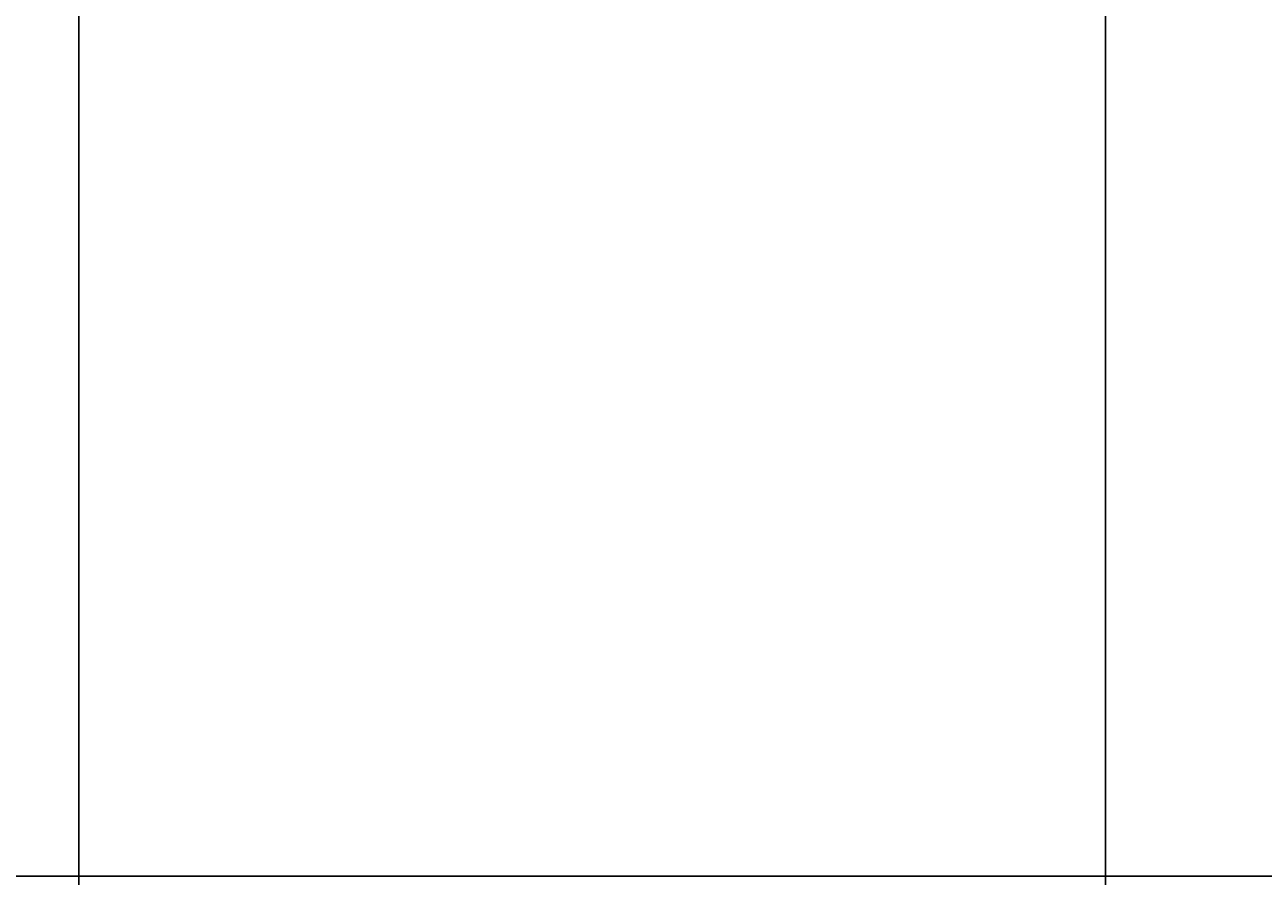
# Model space of a CAD drawing. Units: inches. Extents: x 1998 to 2588, y 1139 to 1977.
# Tile 40 of 134: x 2293 to 2344, y 1523 to 1557. Entities that reach past the tile are written whole.
import ezdxf

# ---------------------------------------------------------------- set-up
doc = ezdxf.new("R2010")
doc.units = ezdxf.units.IN
doc.layers.add('A-ANNO-DIMS', color=2, linetype='Continuous', lineweight=18)
doc.styles.get("Standard").update_dxf_attribs({"font": 'arial.ttf'})
doc.dimstyles.get("Standard").update_dxf_attribs({"dimtxt": 0.18, "dimasz": 0.18, "dimexe": 0.18, "dimexo": 0.0625, "dimgap": 0.09, "dimtad": 0, "dimtih": 1, "dimtoh": 1, "dimdec": 4, "dimzin": 0, "dimdsep": 46, "dimtxsty": 'Standard', "dimcen": 0.09, "dimadec": 0, "dimazin": 0, "dimtfac": 1, "dimtdec": 4, "dimtofl": 0, "dimtmove": 0, "dimatfit": 3, "dimfxl": 1, "dimtolj": 1, "dimtzin": 0, "dimarcsym": 0})

# ---------------------------------------------------------------- blocks, each defined once
blk = doc.blocks.new('*D34')
at = {"layer": 'A-ANNO-DIMS', "color": 0, "lineweight": -2, "transparency": 16777216}
for p, q in [((2407.91, 1594.732), (1997.843, 1594.732)), ((1998.023, 1594.552), (1998.023, 1558.913)), ((1998.023, 1522.912), (1998.023, 1558.552)), ((2407.91, 1522.732), (1997.843, 1522.732))]:
    blk.add_line(p, q, dxfattribs=at)
at = {"layer": 'A-ANNO-DIMS', "color": 0, "transparency": 16777216}
for points in [[(1997.993, 1594.552), (1998.053, 1594.552), (1998.023, 1594.732)], [(1997.993, 1522.912), (1998.053, 1522.912), (1998.023, 1522.732)]]:
    blk.add_solid(points, dxfattribs=at)
at = {"layer": 'Defpoints', "color": 0, "transparency": 16777216}
for p in [(1998.023, 1594.732), (2407.973, 1594.732), (2407.973, 1522.732)]:
    blk.add_point(p, dxfattribs=at)
at = {"layer": 'A-ANNO-DIMS', "color": 0, "transparency": 16777216, "insert": (1998.023, 1558.732), "char_height": 0.18, "attachment_point": 5}
blk.add_mtext('\\A1;72', dxfattribs=at)
blk = doc.blocks.new('*D42')
at = {"layer": 'A-ANNO-DIMS', "color": 0, "lineweight": -2, "transparency": 16777216}
for p, q in [((2287.535, 1588.732), (2588.309, 1588.732)), ((2588.129, 1588.552), (2588.129, 1555.914)), ((2588.129, 1522.912), (2588.129, 1555.55)), ((2287.535, 1522.732), (2588.309, 1522.732))]:
    blk.add_line(p, q, dxfattribs=at)
at = {"layer": 'A-ANNO-DIMS', "color": 0, "transparency": 16777216}
for points in [[(2588.099, 1588.552), (2588.159, 1588.552), (2588.129, 1588.732)], [(2588.099, 1522.912), (2588.159, 1522.912), (2588.129, 1522.732)]]:
    blk.add_solid(points, dxfattribs=at)
at = {"layer": 'Defpoints', "color": 0, "transparency": 16777216}
for p in [(2287.473, 1588.732), (2588.129, 1588.732), (2287.473, 1522.732)]:
    blk.add_point(p, dxfattribs=at)
at = {"layer": 'A-ANNO-DIMS', "color": 0, "transparency": 16777216, "insert": (2588.129, 1555.732), "char_height": 0.18, "attachment_point": 5}
blk.add_mtext('\\A1;66', dxfattribs=at)
blk = doc.blocks.new('*D44')
at = {"layer": 'A-ANNO-DIMS', "color": 0, "lineweight": -2, "transparency": 16777216}
for p, q in [((2295.414, 1588.67), (2295.414, 1138.602)), ((2337.287, 1588.67), (2337.287, 1138.602)), ((2295.594, 1138.782), (2315.953, 1138.782)), ((2337.107, 1138.782), (2316.748, 1138.782))]:
    blk.add_line(p, q, dxfattribs=at)
at = {"layer": 'A-ANNO-DIMS', "color": 0, "transparency": 16777216}
for points in [[(2295.594, 1138.812), (2295.594, 1138.752), (2295.414, 1138.782)], [(2337.107, 1138.812), (2337.107, 1138.752), (2337.287, 1138.782)]]:
    blk.add_solid(points, dxfattribs=at)
at = {"layer": 'Defpoints', "color": 0, "transparency": 16777216}
for p in [(2295.414, 1588.732), (2337.287, 1588.732), (2337.287, 1138.782)]:
    blk.add_point(p, dxfattribs=at)
at = {"layer": 'A-ANNO-DIMS', "color": 0, "transparency": 16777216, "insert": (2316.35, 1138.782), "char_height": 0.18, "attachment_point": 5}
blk.add_mtext('\\A1;41.87', dxfattribs=at)

msp = doc.modelspace()

# ---------------------------------------------------------------- dimensions: what is measured, and where the dimension line sits
at = {"layer": 'A-ANNO-DIMS'}
for base, p1, p2, picture, middle in [((1998.0229, 1594.7324), (2407.9729, 1522.7324), (2407.9729, 1594.7324), '*D34', (1998.0229, 1558.7324)), ((2588.1286, 1588.7324), (2287.4729, 1522.7324), (2287.4729, 1588.7324), '*D42', (2588.1286, 1555.7324))]:
    dim = msp.add_linear_dim(base=base, p1=p1, p2=p2, angle=90, dimstyle='Standard', override={"dimdec": 0, "dimlfac": 1, "dimrnd": 0, "dimzin": 0, "dimdsep": 46, "dimlunit": 2}, dxfattribs=at)
    dim.commit()
    dim.dimension.update_dxf_attribs({"geometry": picture, "text_midpoint": middle})
dim = msp.add_linear_dim(base=(2337.2869, 1138.7824), p1=(2295.4138, 1588.7324), p2=(2337.2869, 1588.7324), dimstyle='Standard', override={"dimdec": 2, "dimlfac": 1, "dimrnd": 0, "dimzin": 0, "dimdsep": 46, "dimlunit": 2}, dxfattribs=at)
dim.commit()
dim.dimension.update_dxf_attribs({"geometry": '*D44', "text_midpoint": (2316.3503, 1138.7824)})

doc.saveas('drawing.dxf')
